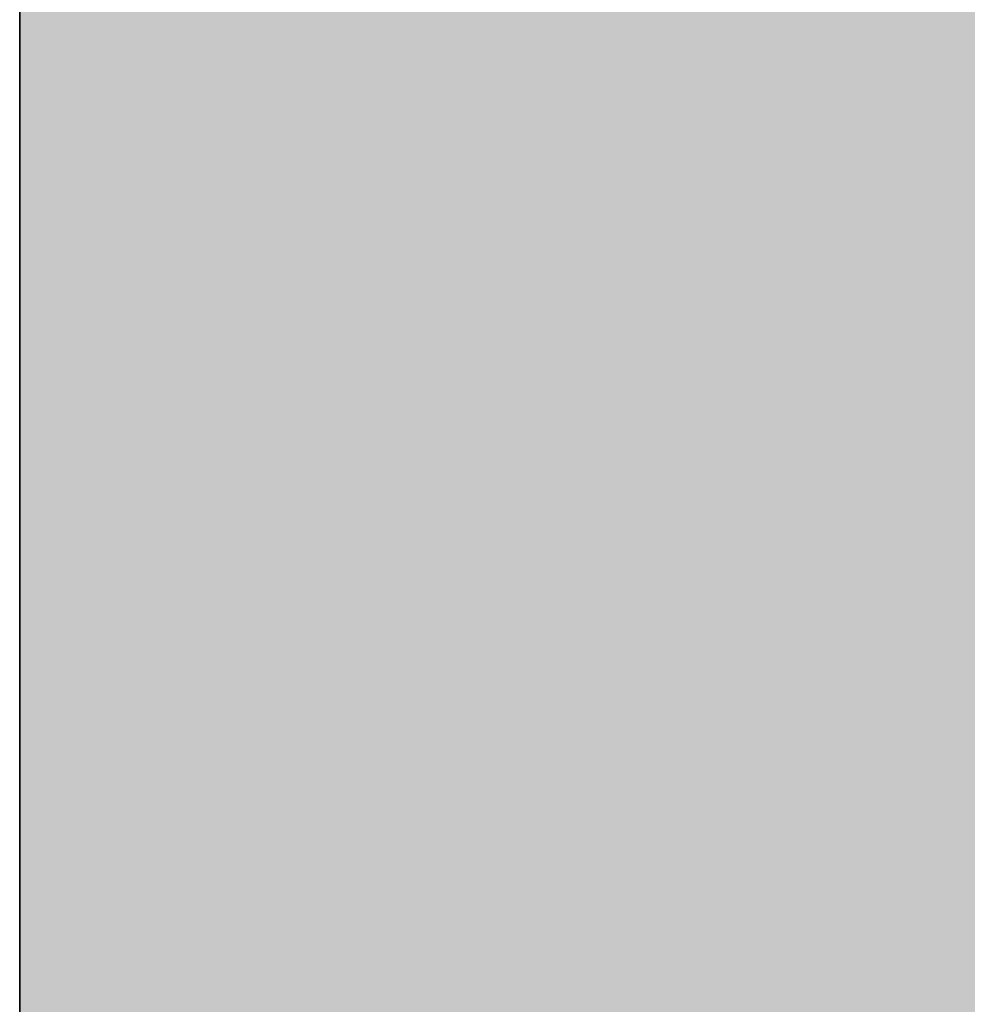
# Model space of a CAD drawing. Units: inches. Extents: x 2091 to 2899, y 967 to 2217.
# Tile 166 of 256: x 2203.143603 to 2203.14684, y 1152.250422 to 1152.253784. Entities that reach past the tile are written whole.
import ezdxf

# ---------------------------------------------------------------- set-up
doc = ezdxf.new("R2010")
doc.units = ezdxf.units.IN
doc.layers.add('A-WALL-PATT', color=141, linetype='Continuous', lineweight=13, true_color=0xadddf7)
doc.layers.add('C-PROP', color=7, linetype='Continuous', lineweight=35)

msp = doc.modelspace()

# ---------------------------------------------------------------- hatches: boundary and pattern name
at = {"layer": 'A-WALL-PATT'}
h = msp.add_hatch(color=256, dxfattribs=at)
h.dxf.hatch_style = 1
h.paths.add_polyline_path([(2803.1436027, 2050.9190588), (2203.1436027, 2050.9190588), (2203.1436027, 1090.9190588), (2803.1436027, 1090.9190588)])
h.paths.add_polyline_path([(2635.7988501, 1147.5404649), (2674.5240524, 1147.5404649, 0.376086), (2678.5296653, 1152.8802017), (2678.5296653, 1159.5564734, 0.333335), (2674.524319, 1163.561846), (2674.524319, 1163.5618504), (2674.524319, 1192.9343904), (2635.8059707, 1192.9343904), (2597.0876225, 1192.9343904), (2597.0876225, 1163.561846, 0.333335), (2593.0822761, 1159.5564734), (2593.0822761, 1152.8802017, 0.376086), (2597.087889, 1147.5404649)], flags=0)
h.paths.add_polyline_path([(2436.0104329, 1278.2407784, 0.000483), (2435.9526433, 1278.215027, -0.001328), (2435.9356253, 1278.1116934, -0.001711), (2436.1164401, 1278.0407583, 0.002185)], flags=0)
h.paths.add_polyline_path([(2794.1436027, 1143.4190588), (2794.1436027, 1347.4190588), (2543.3701706, 1347.4190588), (2543.3701706, 1351.9190588), (2794.1436027, 1351.9190588), (2794.1436027, 1392.7135549), (2793.9473982, 1392.7135549), (2793.9473982, 1473.5368999), (2794.1436027, 1473.5368999), (2794.1436027, 1531.9190588), (2650.1436027, 1531.9190588), (2650.1436027, 1536.4190588), (2794.1436027, 1536.4190588), (2794.1436027, 1692.4190588), (2609.3756095, 1692.4190588), (2609.3756095, 1644.4190588), (2604.8756095, 1644.4190588), (2604.8756095, 1744.9190588), (2609.3756095, 1744.9190588), (2609.3756095, 1696.9190588), (2794.1436027, 1696.9190588), (2794.1436027, 1780.9190588), (2609.6436027, 1780.9190588), (2493.8756095, 1780.9190588), (2493.8756095, 1785.4190588), (2609.6436027, 1785.4190588), (2794.1436027, 1785.4190588), (2794.1436027, 1847.9388214), (2793.9512217, 1847.9388214), (2793.9512217, 1928.7621663), (2794.1436027, 1928.7621663), (2794.1436027, 1941.4190588), (2614.1436027, 1941.4190588), (2614.1436027, 1821.4190588), (2609.6436027, 1821.4190588), (2609.6436027, 1941.4190588), (2392.1436027, 1941.4190588), (2392.1436027, 1819.9190588), (2387.6436027, 1819.9190588), (2387.6436027, 1941.4190588), (2212.1436027, 1941.4190588), (2212.1436027, 1783.9190588), (2392.1436027, 1783.9190588), (2392.1436027, 1780.9190588), (2212.1436027, 1780.9190588), (2212.1436027, 1629.4190588), (2387.6436027, 1629.4190588), (2387.6436027, 1744.9190588), (2392.1436027, 1744.9190588), (2392.1436027, 1627.9190588), (2317.1436027, 1627.9190588), (2317.1436027, 1551.4190588), (2317.1436027, 1536.4190588), (2459.3835909, 1536.4190588), (2459.3835909, 1602.3964802), (2463.8835909, 1602.3964802), (2463.8835909, 1531.9190588), (2456.6436027, 1531.9190588), (2456.6436027, 1529.9190588), (2452.1436027, 1529.9190588), (2452.1436027, 1531.9190588), (2312.6436027, 1531.9190588), (2312.6436027, 1551.4190588), (2306.1436027, 1551.4190588), (2306.1436027, 1555.9190588), (2308.1436027, 1555.9190588), (2308.1436027, 1551.4190588), (2312.6436027, 1551.4190588), (2312.6436027, 1627.9190588), (2212.1436027, 1627.9190588), (2212.1436027, 1555.9190588), (2270.1436027, 1555.9190588), (2270.1436027, 1551.4190588), (2212.1436027, 1551.4190588), (2212.1436027, 1351.9190588), (2272.1436027, 1351.9190588), (2272.1436027, 1347.4190588), (2212.1436027, 1347.4190588), (2212.1436027, 1275.4190588), (2308.1436027, 1275.4190588), (2308.1436027, 1351.9190588), (2452.1436027, 1351.9190588), (2452.1436027, 1493.9190588), (2456.6436027, 1493.9190588), (2456.6436027, 1347.4190588), (2312.6436027, 1347.4190588), (2312.6436027, 1270.9190588), (2212.1436027, 1270.9190588), (2212.1436027, 1099.9190588), (2281.2375229, 1099.9190588), (2282.8710413, 1110.9138034), (2282.0083413, 1116.9966034), (2278.5577413, 1121.4204034), (2268.2056413, 1128.0562034), (2272.0876413, 1128.0562034), (2273.8129413, 1131.9270034), (2279.4203413, 1134.6919034), (2285.0278413, 1135.2449034), (2287.6158413, 1137.4568034), (2288.0471413, 1138.0098034), (2289.3411413, 1140.7747034), (2291.0665413, 1139.6687034), (2292.3605413, 1135.2449034), (2295.3798413, 1136.9038034), (2296.2425413, 1135.7979034), (2297.1052413, 1133.0330034), (2300.1246413, 1138.0098034), (2303.1439413, 1138.0098034), (2304.4379413, 1135.7979034), (2303.1439413, 1133.5860034), (2306.5946413, 1134.6919034), (2307.8887413, 1133.0330034), (2310.9080413, 1135.2449034), (2313.9274413, 1134.1389034), (2315.6268599, 1132.4271023), (2308.3200413, 1117.5496034), (2290.2038413, 1109.8079034), (2288.9098413, 1103.1721034), (2289.2723086, 1099.9190588), (2434.9182274, 1099.9190588), (2431.5932274, 1124.7880588), (2429.9302274, 1169.5530588), (2430.9271848, 1240.5196942), (2435.6589255, 1238.1861258), (2437.1352274, 1196.5540588), (2438.7982274, 1143.9730588), (2442.6782274, 1111.9980588), (2446.5582274, 1099.9190588), (2794.1436027, 1099.9190588), (2794.1436027, 1138.9190588), (2548.0324471, 1138.9190588), (2548.0324471, 1143.4190588), (2548.0324471, 1148.8190588), (2546.6684571, 1148.0315588), (2528.6856919, 1179.1786218, 0.256256), (2512.0324471, 1148.8190588), (2512.0324471, 1143.4190588), (2512.0324471, 1138.9190588), (2507.5324471, 1138.9190588), (2507.5324471, 1143.4190588), (2507.5324471, 1148.8190588, 0.256256), (2490.8792023, 1179.1786218), (2472.8964371, 1148.0315588), (2471.5324471, 1148.8190588), (2471.5324471, 1143.4190588), (2467.0324471, 1143.4190588), (2467.0324471, 1269.9457858, 0.039061), (2460.9099871, 1273.5800588), (2467.0324471, 1273.5800588), (2467.0324471, 1286.3253638, 0.014511), (2465.2161944, 1286.7619052), (2467.0324471, 1287.0525761), (2467.0324471, 1323.4190588), (2471.5324471, 1323.4190588), (2471.5324471, 1148.8190588), (2489.5324471, 1179.9959734), (2490.8964371, 1179.2084734), (2490.8792023, 1179.1786218, -0.256256), (2507.5324471, 1148.8190588), (2507.5324471, 1143.4190588), (2512.0324471, 1143.4190588), (2512.0324471, 1148.8190588, -0.256256), (2528.6856919, 1179.1786218), (2528.6684571, 1179.2084734), (2530.0324471, 1179.9959734), (2548.0324471, 1148.8190588), (2548.0324471, 1143.4190588)], flags=16)
h.paths.add_polyline_path([(2607.7685461, 1200.9450832), (2607.7685461, 1265.0306251), (2597.0876225, 1281.0520106), (2619.7845852, 1281.0520106), (2627.795278, 1337.1268598), (2635.7988501, 1337.1268598), (2643.8166634, 1337.1268598), (2651.8273562, 1281.0520106), (2674.524319, 1281.0520106), (2663.8433953, 1265.0306251), (2663.8433953, 1200.9450832), (2635.8059707, 1200.9450832)], flags=0)
edge = h.paths.add_edge_path(flags=0)
edge.add_ellipse((13303.8962153, 1272.9987247), major_axis=(-10595.3130399, 0.0000005), ratio=0.842303870086, start_angle=0.62823721906, end_angle=0.64655409989, ccw=False)
edge.add_ellipse((2711.7004495, 1156.8526781), major_axis=(2.2197691, 0), ratio=0.84230387, start_angle=111.5352435, end_angle=180.6282372, ccw=False)
edge.add_ellipse((13303.1562922, 1272.9987246), major_axis=(-10593.0263064, 0), ratio=0.842303869544, start_angle=0.52827147182, end_angle=0.64655409706, ccw=False)
edge.add_line((2710.7645961, 1175.3332951), (2710.1299858, 1175.3332951))
edge.add_ellipse((2710.1299858, 1176.5797752), major_axis=(1.4798461, 0), ratio=0.84230387, start_angle=180, end_angle=270, ccw=False)
edge.add_line((2708.6501397, 1176.5797752), (2708.6501397, 1200.7829144))
edge.add_ellipse((2710.1299858, 1200.7829144), major_axis=(1.4798461, 0), ratio=0.84230387, start_angle=90, end_angle=180, ccw=False)
edge.add_line((2710.1299858, 1202.0293944), (2710.4650752, 1202.0293944))
edge.add_ellipse((13303.1562922, 1272.9987246), major_axis=(-10593.0263064, 0), ratio=0.842303869544, start_angle=-0.09022908859, end_angle=0.38386677879, ccw=False)
edge.add_ellipse((2710.1299858, 1290.9270308), major_axis=(-1.4798461, 0), ratio=0.84230387, start_angle=0, end_angle=90, ccw=False)
edge.add_line((2708.6501397, 1290.9270308), (2708.6501397, 1315.13017))
edge.add_ellipse((2710.1299858, 1315.13017), major_axis=(-1.4798461, 0), ratio=0.84230387, start_angle=-90, end_angle=0, ccw=False)
edge.add_line((2710.1299858, 1316.3766501), (2710.7063141, 1316.3766501))
edge.add_ellipse((3238.4017202, 1296.2895655), major_axis=(528.2339998, 0), ratio=0.84230386954, start_angle=176.349572414, end_angle=177.820049686, ccw=False)
edge.add_ellipse((2775.0630432, 1071.4506962), major_axis=(313.3077613, 0), ratio=0.84230386954, start_angle=102.125965552, end_angle=103.780528989, ccw=False)
edge.add_ellipse((2775.0630432, 1078.3056979), major_axis=(-305.3028915, 0), ratio=0.84230386955, start_angle=-79.790461003, end_angle=-77.555372706, ccw=False)
edge.add_ellipse((2695.1417666, 1541.9753825), major_axis=(-250.9602162, 0), ratio=0.84230386954, start_angle=99.256566007, end_angle=102.554932644)
edge.add_line((2741.4103262, 1334.2142554), (2747.1325454, 1337.3784768))
edge.add_ellipse((2747.5386163, 1336.8574776), major_axis=(-0.739923, 0), ratio=0.84230387, start_angle=270, end_angle=307.9331305, ccw=False)
edge.add_ellipse((2747.5386163, 1336.8574776), major_axis=(-0.739923, 0), ratio=0.84230387, start_angle=232.0668695, end_angle=270, ccw=False)
edge.add_line((2747.9446872, 1337.3784768), (2753.6669064, 1334.2142554))
edge.add_ellipse((2799.935466, 1541.9753825), major_axis=(250.9602162, 0), ratio=0.84230386954, start_angle=257.445067356, end_angle=260.743433993)
edge.add_ellipse((2720.0141894, 1078.3056979), major_axis=(305.3028915, 0), ratio=0.84230386954, start_angle=77.555372707, end_angle=79.790461003, ccw=False)
edge.add_ellipse((2720.0141894, 1071.4506962), major_axis=(-313.3077613, 0), ratio=0.84230386954, start_angle=256.219471011, end_angle=257.874034448, ccw=False)
edge.add_ellipse((2256.6755124, 1296.2895655), major_axis=(-528.2339998, 0), ratio=0.84230386954, start_angle=182.179950314, end_angle=183.650427586, ccw=False)
edge.add_line((2784.3709184, 1316.3766501), (2784.9472468, 1316.3766501))
edge.add_ellipse((2784.9472468, 1315.13017), major_axis=(1.4798461, 0), ratio=0.84230387, start_angle=0, end_angle=90, ccw=False)
edge.add_line((2786.4270928, 1315.13017), (2786.4270928, 1290.9270308))
edge.add_ellipse((2784.9472468, 1290.9270308), major_axis=(1.4798461, 0), ratio=0.84230387, start_angle=270, end_angle=360, ccw=False)
edge.add_ellipse((-7808.0790596, 1272.9987246), major_axis=(10593.0263063, 0), ratio=0.842303869544, start_angle=-0.38386677879, end_angle=0.09022908859, ccw=False)
edge.add_line((2784.6121574, 1202.0293944), (2784.9472468, 1202.0293944))
edge.add_ellipse((2784.9472468, 1200.7829144), major_axis=(1.4798461, 0), ratio=0.84230387, start_angle=0, end_angle=90, ccw=False)
edge.add_line((2786.4270928, 1200.7829144), (2786.4270928, 1176.5797752))
edge.add_ellipse((2784.9472468, 1176.5797752), major_axis=(-1.4798461, 0), ratio=0.84230387, start_angle=90, end_angle=180, ccw=False)
edge.add_line((2784.9472468, 1175.3332951), (2784.3126365, 1175.3332951))
edge.add_ellipse((-7808.0790596, 1272.9987246), major_axis=(10593.0263063, 0), ratio=0.842303869544, start_angle=-0.61864319632, end_angle=-0.52827147182, ccw=False)
edge.add_ellipse((2783.3767831, 1156.8526781), major_axis=(-2.2197691, 0), ratio=0.84230387, start_angle=179.3717628, end_angle=248.4647566, ccw=False)
edge.add_ellipse((-7808.8189826, 1272.9987246), major_axis=(-10595.3130398, 0.0000036), ratio=0.842303865762, start_angle=179.3534459226, end_angle=179.37176280343, ccw=False)
edge.add_ellipse((2780.2973026, 1153.500793), major_axis=(-5.2464256, 0), ratio=0.84230387, start_angle=90, end_angle=179.3534459, ccw=False)
edge.add_line((2780.2973026, 1149.0817084), (2714.77993, 1149.0817084))
edge.add_ellipse((2714.77993, 1153.500793), major_axis=(5.2464256, 0), ratio=0.84230387, start_angle=180.6465541, end_angle=270, ccw=False)
edge = h.paths.add_edge_path(flags=0)
edge.add_line((2718.1873674, 1151.0078329), (2718.1873674, 1170.4723638))
edge.add_ellipse((2721.1470595, 1170.4723638), major_axis=(-2.9596921, 0), ratio=0.84230387, start_angle=-90, end_angle=0, ccw=False)
edge.add_line((2721.1470595, 1172.965324), (2773.9301731, 1172.965324))
edge.add_ellipse((2773.9301731, 1170.4723638), major_axis=(-2.9596921, 0), ratio=0.84230387, start_angle=180, end_angle=270, ccw=False)
edge.add_line((2776.8898652, 1170.4723638), (2776.8898652, 1151.0078329))
edge.add_line((2776.8898652, 1151.0078329), (2718.1873674, 1151.0078329))
edge = h.paths.add_edge_path(flags=0)
edge.add_line((2718.1873674, 1180.2341502), (2718.1873674, 1199.0578342))
edge.add_ellipse((2747.5386163, 1320.3986402), major_axis=(147.0179239, 0), ratio=0.84230386954, start_angle=256.40186531, end_angle=283.59813469)
edge.add_line((2776.8898652, 1199.0578342), (2776.8898652, 1180.2341502))
edge.add_ellipse((2747.5386163, 1301.5749562), major_axis=(147.0179239, 0), ratio=0.84230386954, start_angle=256.40186531, end_angle=283.59813469, ccw=False)
edge = h.paths.add_edge_path(flags=0)
edge.add_ellipse((13303.1562922, 1272.9987246), major_axis=(-10591.5464603, 0), ratio=0.842303869555, start_angle=0.05559431352, end_angle=0.37776419393, ccw=False)
edge.add_line((2711.6168595, 1262.7217103), (2715.6674076, 1249.4953957))
edge.add_ellipse((6413.8919626, 1241.691919), major_axis=(-3698.2361592, 0), ratio=0.842303869547, start_angle=-0.120897369, end_angle=0.3640763489)
edge.add_line((2715.7610383, 1218.1924547), (2711.9343065, 1203.167361))
edge = h.paths.add_edge_path(flags=0)
edge.add_line((2718.1873674, 1251.074566), (2716.0024854, 1267.4504351))
edge.add_ellipse((2742.1511746, 1202.1895399), major_axis=(81.7725845, 0), ratio=0.8423038695, start_angle=94.277420963, end_angle=111.834953797, ccw=False)
edge.add_line((2737.0097482, 1270.9306255), (2758.0674844, 1270.9306255))
edge.add_ellipse((2752.926058, 1202.1895399), major_axis=(81.7725845, 0), ratio=0.8423038695, start_angle=68.165046203, end_angle=85.722579037, ccw=False)
edge.add_line((2779.0747472, 1267.4504351), (2776.8898652, 1251.074566))
edge.add_ellipse((2750.3380588, 1187.8853558), major_axis=(79.5796641, 0), ratio=0.8423038695, start_angle=67.208085122, end_angle=85.129930403)
edge.add_line((2756.0346562, 1254.7436557), (2739.0425764, 1254.7436557))
edge.add_ellipse((2744.7391738, 1187.8853558), major_axis=(79.5796641, 0), ratio=0.8423038695, start_angle=94.870069597, end_angle=112.791914878)
edge = h.paths.add_edge_path(flags=0)
edge.add_line((2783.1429261, 1203.167361), (2779.3161943, 1218.1924547))
edge.add_ellipse((-918.81473, 1241.691919), major_axis=(3698.2361592, 0), ratio=0.842303869546, start_angle=-0.3640763489, end_angle=0.120897369)
edge.add_line((2779.409825, 1249.4953957), (2783.4603731, 1262.7217103))
edge.add_ellipse((-7808.0790596, 1272.9987246), major_axis=(-10591.5464603, 0), ratio=0.84230386954, start_angle=179.6222358061, end_angle=179.94440568651, ccw=False)
edge = h.paths.add_edge_path(flags=0)
edge.add_ellipse((2734.2008921, 1286.6904402), major_axis=(-0.3566086, 6.3400775), ratio=0.603833576, start_angle=89.00201428, end_angle=253.65740805, ccw=False)
edge.add_line((2730.3690013, 1286.5418057), (2730.3690013, 1301.3519803))
edge.add_line((2730.3690013, 1301.3519803), (2735.9133107, 1305.2148028))
edge.add_ellipse((2736.3849168, 1304.7345612), major_axis=(0.739923, 0), ratio=0.84230387, start_angle=90, end_angle=134.4802109, ccw=False)
edge.add_line((2736.3849168, 1305.3578013), (2738.0327829, 1305.3578013))
edge.add_line((2738.0327829, 1305.3578013), (2738.0327829, 1307.7079274))
edge.add_ellipse((2794.201642, 1307.7079274), major_axis=(56.168859, 0), ratio=0.8423038695, start_angle=150.5614304, end_angle=180, ccw=False)
edge.add_ellipse((2700.8755906, 1307.7079274), major_axis=(-56.168859, 0), ratio=0.8423038695, start_angle=180, end_angle=209.4385696, ccw=False)
edge.add_line((2757.0444497, 1307.7079274), (2757.0444497, 1305.3578013))
edge.add_line((2757.0444497, 1305.3578013), (2758.6923157, 1305.3578013))
edge.add_ellipse((2758.6923157, 1304.7345612), major_axis=(-0.739923, 0), ratio=0.84230387, start_angle=225.5197891, end_angle=270, ccw=False)
edge.add_line((2759.1639219, 1305.2148028), (2764.7082312, 1301.3519803))
edge.add_line((2764.7082312, 1301.3519803), (2764.7082312, 1286.5418057))
edge.add_ellipse((2760.8763405, 1286.6904402), major_axis=(0.3566086, 6.3400775), ratio=0.603833576, start_angle=106.34259195, end_angle=270.99798572, ccw=False)
edge.add_line((2757.0444497, 1285.7970896), (2757.0444497, 1307.7079274))
edge.add_ellipse((2700.8755906, 1307.7079274), major_axis=(-56.168859, 0), ratio=0.8423038695, start_angle=180, end_angle=209.4385696)
edge.add_ellipse((2794.201642, 1307.7079274), major_axis=(56.168859, 0), ratio=0.8423038695, start_angle=150.5614304, end_angle=180)
edge.add_line((2738.0327829, 1307.7079274), (2738.0327829, 1285.7970896))
h.paths.add_polyline_path([(2417.8122727, 1104.449704), (2413.4922727, 1102.529704), (2410.6122727, 1103.969704), (2409.1722727, 1106.369704), (2407.2522727, 1107.329704), (2406.2922727, 1109.729704), (2405.3322727, 1114.049704), (2405.3322727, 1117.889704), (2406.2922727, 1120.129704), (2407.2522727, 1119.809704), (2408.8483218, 1118.3276585), (2410.1739451, 1119.4241703), (2410.2112727, 1120.405704), (2411.0407305, 1121.4190541), (2410.6992727, 1119.858704), (2410.1739451, 1119.4241703), (2410.0884515, 1117.1761095), (2411.1328361, 1116.2063237), (2413.9722727, 1119.329704), (2416.8522727, 1120.769704), (2416.8697209, 1120.7987842), (2417.0350713, 1119.4051162), (2417.8962134, 1118.1433844), (2418.2922727, 1118.369704), (2419.5444467, 1120.0392692), (2419.3609153, 1118.387487), (2419.0321078, 1119.3561507), (2418.3989394, 1118.5119262), (2419.2522727, 1114.529704), (2418.7940909, 1107.1987949)], flags=0)
h.paths.add_polyline_path([(2508.8701706, 1347.4190588), (2508.3701706, 1347.4190588), (2508.3701706, 1351.9190588), (2508.8701706, 1351.9190588)], flags=0)
h.paths.add_polyline_path([(2473.3701706, 1347.4190588), (2472.3701706, 1347.4190588), (2467.8701706, 1347.4190588), (2467.8701706, 1455.4190588), (2472.3701706, 1455.4190588), (2472.3701706, 1352.4190588), (2473.3701706, 1352.4190588)], flags=0)
h.paths.add_polyline_path([(2352.106244, 1217.4461971), (2349.226244, 1218.8861971), (2347.786244, 1221.2861971), (2345.866244, 1222.2461971), (2344.906244, 1224.6461971), (2343.946244, 1228.9661971), (2343.946244, 1232.8061971), (2344.906244, 1235.0461971), (2345.866244, 1234.7261971), (2347.4622931, 1233.2441515), (2348.7879164, 1234.3406634), (2348.825244, 1235.3221971), (2349.6547018, 1236.3355471), (2349.313244, 1234.7751971), (2348.7879164, 1234.3406634), (2348.7024228, 1232.0926025), (2349.7468074, 1231.1228168), (2352.586244, 1234.2461971), (2355.466244, 1235.6861971), (2355.4836921, 1235.7152773), (2355.6490426, 1234.3216093), (2356.5101846, 1233.0598774), (2356.906244, 1233.2861971), (2358.1584179, 1234.9557623), (2357.9748866, 1233.3039801), (2357.6460791, 1234.2726438), (2357.0129107, 1233.4284193), (2357.866244, 1229.4461971), (2357.4080622, 1222.115288), (2356.426244, 1219.3661971)], flags=0)
h.paths.add_polyline_path([(2348.2967999, 1112.2244204), (2347.0137999, 1112.3104204), (2345.5297999, 1114.1274204), (2345.7317999, 1115.8584204), (2346.8117999, 1116.9824204), (2346.8117999, 1114.6464204), (2345.8667999, 1114.2144204), (2346.8797999, 1114.3004204)], flags=0)
h.paths.add_polyline_path([(2347.0137999, 1110.9264204), (2346.2717999, 1110.4934204), (2346.6097999, 1111.1864204)], flags=0)
h.paths.add_polyline_path([(2345.8667999, 1118.1944204), (2345.5297999, 1117.3294204), (2343.7077999, 1118.0214204), (2344.3827999, 1118.6264204)], flags=0)
h.paths.add_polyline_path([(2346.6767999, 1109.2824204), (2346.0697999, 1108.0714204), (2345.8667999, 1110.0614204)], flags=0)
h.paths.add_polyline_path([(2345.0567999, 1119.7514204), (2343.6397999, 1119.7514204), (2343.9777999, 1121.1354204)], flags=0)
h.paths.add_polyline_path([(2345.2597999, 1116.5504204), (2345.1247999, 1115.8584204), (2344.9217999, 1115.6854204), (2344.7197999, 1116.3774204)], flags=0)
h.paths.add_polyline_path([(2345.6647999, 1112.3104204), (2345.4617999, 1111.5324204), (2344.0447999, 1111.9644204), (2344.6517999, 1112.5704204)], flags=0)
h.paths.add_polyline_path([(2345.1917999, 1113.3494204), (2344.4497999, 1113.8684204), (2344.7197999, 1114.3874204)], flags=0)
h.paths.add_polyline_path([(2344.6517999, 1116.8094204), (2344.1797999, 1115.6854204), (2344.6517999, 1115.3394204), (2343.9097999, 1114.9064204), (2343.0327999, 1115.9444204), (2343.6397999, 1116.4634204)], flags=0)
h.paths.add_polyline_path([(2345.8667999, 1106.6864204), (2344.9897999, 1105.5624204), (2344.5167999, 1106.6004204)], flags=0)
h.paths.add_polyline_path([(2344.8547999, 1110.0614204), (2344.5167999, 1109.2824204), (2344.1127999, 1109.7154204)], flags=0)
h.paths.add_polyline_path([(2344.0447999, 1113.5224204), (2343.4377999, 1113.0894204), (2342.7627999, 1113.9544204)], flags=0)
h.paths.add_polyline_path([(2344.3147999, 1111.0124204), (2342.9647999, 1110.3204204), (2342.9647999, 1111.0994204)], flags=0)
h.paths.add_polyline_path([(2345.1247999, 1104.6974204), (2344.5847999, 1103.7454204), (2344.4497999, 1104.2644204)], flags=0)
h.paths.add_polyline_path([(2342.8297999, 1121.2224204), (2341.7497999, 1120.5304204), (2340.5357999, 1121.0494204), (2340.1307999, 1121.8284204), (2340.6707999, 1122.9524204), (2341.1427999, 1121.8284204), (2341.6147999, 1122.0014204)], flags=0)
h.paths.add_polyline_path([(2342.9647999, 1119.7514204), (2343.0327999, 1118.4534204), (2342.0877999, 1118.0214204), (2342.0197999, 1119.4914204)], flags=0)
h.paths.add_polyline_path([(2342.6947999, 1116.8964204), (2341.9527999, 1116.6364204), (2342.0197999, 1117.3294204)], flags=0)
h.paths.add_polyline_path([(2343.0327999, 1112.2244204), (2342.0197999, 1111.7914204), (2341.5477999, 1112.2244204), (2342.3577999, 1113.3494204)], flags=0)
h.paths.add_polyline_path([(2343.7747999, 1104.4374204), (2342.6277999, 1102.8804204), (2342.6947999, 1104.6104204), (2343.4377999, 1105.1294204)], flags=0)
h.paths.add_polyline_path([(2342.0197999, 1115.0794204), (2340.8057999, 1115.5124204), (2340.9407999, 1116.3774204)], flags=0)
h.paths.add_polyline_path([(2341.4807999, 1120.0974204), (2341.4807999, 1119.4054204), (2341.0757999, 1119.5784204), (2341.1427999, 1120.0974204)], flags=0)
h.paths.add_polyline_path([(2341.8177999, 1114.4734204), (2340.9407999, 1113.0894204), (2340.8057999, 1114.5604204)], flags=0)
h.paths.add_polyline_path([(2341.1427999, 1118.5404204), (2340.9407999, 1116.9824204), (2339.0507999, 1117.6754204), (2339.0507999, 1118.6264204)], flags=0)
h.paths.add_polyline_path([(2342.6947999, 1101.6684204), (2341.9527999, 1101.8414204), (2342.5597999, 1102.3614204)], flags=0)
h.paths.add_polyline_path([(2340.3327999, 1119.6654204), (2338.4437999, 1119.5784204), (2337.9037999, 1120.3574204), (2339.6577999, 1120.6164204)], flags=0)
h.paths.add_polyline_path([(2340.3327999, 1115.3394204), (2340.0627999, 1113.6954204), (2339.3877999, 1115.3394204)], flags=0)
h.paths.add_polyline_path([(2341.8177999, 1103.8314204), (2341.5477999, 1102.8804204), (2341.1427999, 1103.6584204)], flags=0)
h.paths.add_polyline_path([(2339.0507999, 1122.8664204), (2337.2957999, 1121.8284204), (2337.0937999, 1123.1254204), (2337.7687999, 1123.8184204)], flags=0)
h.paths.add_polyline_path([(2339.1177999, 1121.7414204), (2338.8477999, 1121.2224204), (2338.1737999, 1121.0494204), (2338.3757999, 1121.5684204)], flags=0)
h.paths.add_polyline_path([(2339.1857999, 1119.3194204), (2338.6457999, 1118.7134204), (2338.2407999, 1118.1074204), (2338.2407999, 1118.8864204)], flags=0)
h.paths.add_polyline_path([(2341.1427999, 1101.9284204), (2340.6027999, 1101.2364204), (2340.0627999, 1101.8414204), (2340.6027999, 1102.3614204)], flags=0)
h.paths.add_polyline_path([(2337.6337999, 1117.7614204), (2336.6207999, 1118.2804204), (2337.2957999, 1118.9724204)], flags=0)
h.paths.add_polyline_path([(2336.8237999, 1119.5784204), (2334.7987999, 1118.9724204), (2335.2037999, 1120.3574204), (2336.5537999, 1120.8764204)], flags=0)
h.paths.add_polyline_path([(2339.1177999, 1100.4574204), (2337.3637999, 1100.5434204), (2336.7557999, 1101.2364204)], flags=0)
h.paths.add_polyline_path([(2336.3507999, 1122.4334204), (2336.0137999, 1121.9144204), (2334.9337999, 1122.4334204), (2334.5287999, 1123.4714204), (2335.7437999, 1122.7794204)], flags=0)
h.paths.add_polyline_path([(2334.7317999, 1120.8764204), (2334.2587999, 1120.3574204), (2334.0567999, 1120.7894204), (2334.5967999, 1121.3084204)], flags=0)
h.paths.add_polyline_path([(2334.4617999, 1122.1744204), (2332.5717999, 1121.3084204), (2331.3567999, 1122.1744204), (2332.0997999, 1122.8664204)], flags=0)
h.paths.add_polyline_path([(2334.2587999, 1118.5404204), (2333.3817999, 1118.4534204), (2333.6517999, 1119.3194204)], flags=0)
h.paths.add_polyline_path([(2335.5417999, 1102.2744204), (2334.1917999, 1102.6204204), (2335.2717999, 1103.3124204)], flags=0)
h.paths.add_polyline_path([(2332.7067999, 1119.6654204), (2331.6947999, 1120.4434204), (2332.5047999, 1120.7894204)], flags=0)
h.paths.add_polyline_path([(2334.7317999, 1101.1494204), (2333.5167999, 1101.5824204), (2333.9887999, 1101.7554204)], flags=0)
h.paths.add_polyline_path([(2332.6397999, 1116.6364204), (2331.0867999, 1116.2904204), (2331.9647999, 1118.1944204)], flags=0)
h.paths.add_polyline_path([(2330.7497999, 1121.5684204), (2330.2767999, 1120.2704204), (2328.5227999, 1119.3194204), (2328.9947999, 1121.0494204)], flags=0)
h.paths.add_polyline_path([(2330.7497999, 1118.6264204), (2330.0077999, 1117.5024204), (2329.8727999, 1118.0214204)], flags=0)
h.paths.add_polyline_path([(2332.0997999, 1102.3614204), (2330.5467999, 1102.0144204), (2331.6947999, 1102.9664204)], flags=0)
h.paths.add_polyline_path([(2329.5347999, 1113.6084204), (2329.0627999, 1112.3104204), (2328.5897999, 1113.3494204)], flags=0)
h.paths.add_polyline_path([(2328.3877999, 1117.8484204), (2327.5097999, 1116.5504204), (2327.1727999, 1117.7614204)], flags=0)
h.paths.add_polyline_path([(2329.7377999, 1106.5134204), (2329.5347999, 1105.3024204), (2328.2527999, 1106.0814204)], flags=0)
h.paths.add_polyline_path([(2328.6577999, 1114.3874204), (2328.0497999, 1114.1274204), (2328.3197999, 1114.9064204)], flags=0)
h.paths.add_polyline_path([(2328.3197999, 1112.2244204), (2327.1057999, 1112.1374204), (2326.7007999, 1112.6564204)], flags=0)
h.paths.add_polyline_path([(2326.9027999, 1115.2524204), (2326.7007999, 1114.1274204), (2325.2157999, 1113.6084204), (2326.0927999, 1115.3394204)], flags=0)
h.paths.add_polyline_path([(2326.6327999, 1108.3304204), (2326.0927999, 1107.3794204), (2325.8907999, 1108.5034204), (2326.4977999, 1109.1094204)], flags=0)
h.paths.add_polyline_path([(2615.1436027, 1531.9190588), (2609.6436027, 1531.9190588), (2609.6436027, 1620.4190588), (2614.1436027, 1620.4190588), (2614.1436027, 1536.4190588), (2615.1436027, 1536.4190588)], flags=0)
h.paths.add_polyline_path([(2545.1436027, 1563.4190588), (2464.1436027, 1563.4190588), (2464.1436027, 1632.4190588), (2509.1436027, 1632.4190588), (2509.1436027, 1627.9190588), (2509.1436027, 1603.9190588), (2468.6436027, 1603.9190588), (2468.6436027, 1567.9190588), (2540.6436027, 1567.9190588), (2540.6436027, 1591.9190588), (2545.1436027, 1591.9190588)], flags=0)
h.paths.add_polyline_path([(2388.9690483, 1549.985735), (2357.4341811, 1549.985735), (2357.4341811, 1623.3607783), (2399.3627772, 1623.3607783), (2435.6894654, 1623.3607783), (2435.5925469, 1602.5592734), (2435.5925469, 1602.3964802), (2388.9690483, 1602.3964802)], flags=0)
h.paths.add_polyline_path([(2388.8806282, 1555.8091511), (2374.9044295, 1555.8091511), (2374.9044295, 1600.5715641), (2374.9044295, 1615.4576454), (2406.3508766, 1615.4576454), (2406.3508766, 1618.9394309), (2412.1742927, 1615.4576454), (2406.3508766, 1611.9758599), (2406.3508766, 1615.4576454), (2388.8806282, 1615.4576454)], flags=0)
h.paths.add_polyline_path([(2568.8756095, 1644.4190588), (2453.3756095, 1644.4190588), (2453.3756095, 1785.4190588), (2457.8756095, 1785.4190588), (2457.8756095, 1648.9190588), (2568.8756095, 1648.9190588)], flags=0)
h.paths.add_polyline_path([(2212.1436027, 1945.9190588), (2212.1436027, 2041.9190588), (2794.1436027, 2041.9190588), (2794.1436027, 1945.9190588)], flags=16)
h.paths.add_polyline_path([(2271.0827276, 1964.3172377), (2776.852968, 1964.3172377), (2776.852968, 2037.1696226), (2271.0827276, 2037.1696226)], flags=8)
h.paths.add_polyline_path([(2380.6492852, 1536.8241435), (2461.0408087, 1536.8241435), (2461.0408087, 1554.6525871), (2380.6492852, 1554.6525871)], flags=8)
h.paths.add_polyline_path([(2240.7557092, 1609.7254508), (2309.1858294, 1609.7254508), (2309.1858294, 1617.6982037), (2240.7557092, 1617.6982037)], flags=8)
h.paths.add_polyline_path([(2212.6772554, 1313.5041021), (2282.5915203, 1313.5041021), (2282.5915203, 1322.7452389), (2212.6772554, 1322.7452389)], flags=8)
h.paths.add_polyline_path([(2457.111976, 1114.778574), (2558.4815807, 1114.778574), (2558.4815807, 1142.2196823), (2457.111976, 1142.2196823)], flags=8)
h.paths.add_polyline_path([(2473.4423372, 1273.0100672), (2604.6412257, 1273.0100672), (2604.6412257, 1318.3469349), (2473.4423372, 1318.3469349)], flags=8)
h.paths.add_polyline_path([(2638.8763024, 1626.9774316), (2684.2503675, 1627.9767377), (2684.0384825, 1637.5974944), (2638.6644174, 1636.5981884)], flags=8)
h.paths.add_polyline_path([(2537.5905538, 1453.7934466), (2628.3895472, 1453.7934466), (2628.3895472, 1475.3448114), (2537.5905538, 1475.3448114)], flags=8)
h.paths.add_polyline_path([(2504.1376376, 1714.6323972), (2554.6471875, 1714.6323972), (2554.6471875, 1730.2377115), (2504.1376376, 1730.2377115)], flags=8)
h.paths.add_polyline_path([(2487.5011806, 1575.6518716), (2535.0971214, 1575.6518716), (2535.0971214, 1598.3776456), (2487.5011806, 1598.3776456)], flags=8)
h.paths.add_polyline_path([(2709.0994004, 1735.7102784), (2740.0166009, 1735.7102784), (2740.0166009, 1749.9376406), (2709.0994004, 1749.9376406)], flags=8)
h.paths.add_polyline_path([(2442.4384239, 1792.1716575), (2564.7288353, 1792.1716575), (2564.7288353, 1842.0001626), (2442.4384239, 1842.0001626)], flags=8)
h.paths.add_polyline_path([(2655.8158012, 1809.6440763), (2789.5201425, 1806.6937963), (2790.0849768, 1832.2916379), (2656.3806355, 1835.2419179)], flags=8)
h.paths.add_polyline_path([(2234.8426972, 1797.7201432), (2368.5928512, 1794.7688523), (2369.1607182, 1820.504132), (2235.4105642, 1823.4554229)], flags=8)
h.paths.add_polyline_path([(2245.1384659, 1644.0063348), (2398.4277329, 1640.6238997), (2398.9948417, 1666.3248199), (2245.7055747, 1669.7072549)], flags=8)
h.paths.add_polyline_path([(2306.1428474, 1431.1685186), (2413.7683138, 1428.7936873), (2414.3331481, 1454.3915289), (2306.7076817, 1456.7663602)], flags=8)
h.paths.add_polyline_path([(2306.834582, 1458.2331447), (2393.3804836, 1456.3234487), (2393.9328082, 1481.3543583), (2307.3869066, 1483.2640542)], flags=8)

# ---------------------------------------------------------------- linework, layer by layer
at = {"layer": 'C-PROP'}
msp.add_lwpolyline([(2203.1436027, 2050.9190588), (2803.1436027, 2050.9190588), (2803.1436027, 1090.9190588), (2203.1436027, 1090.9190588)], close=True, dxfattribs=at)

doc.saveas('drawing.dxf')
